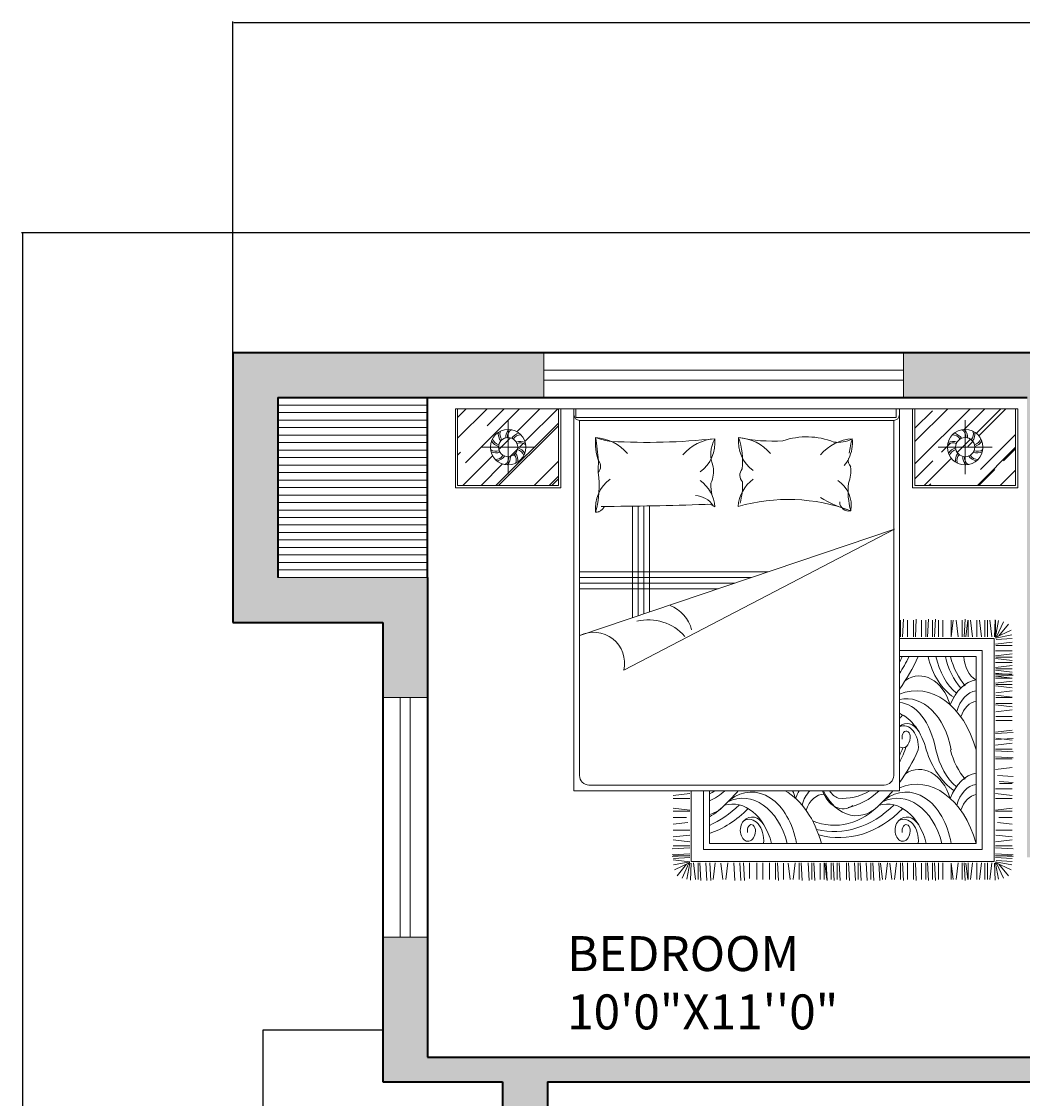
# Model space of a CAD drawing. Units: inches. Extents: x 2540 to 3167, y 3083 to 4007.
# Tile 12 of 15: x 2540 to 2741, y 3791 to 4007. Entities that reach past the tile are written whole.
import ezdxf

# ---------------------------------------------------------------- set-up
doc = ezdxf.new("R2010")
doc.units = ezdxf.units.IN
for name, color, linetype, lineweight in [('A-ANNO-DIMS', 2, 'Continuous', 18), ('A-AREA-IDEN', 7, 'Continuous', 18), ('A-FLOR-EDGE', 7, 'Continuous', 25), ('A-FLOR-PATT', 8, 'Continuous', 13), ('A-FURN', 8, 'Continuous', 13), ('A-GLAZ', 4, 'Continuous', 18)]:
    doc.layers.add(name, color=color, linetype=linetype, lineweight=lineweight)
doc.layers.add('A-WALL', color=143, linetype='Continuous', lineweight=35, true_color=0x7aafdf)
doc.layers.add('A-WALL-PATT', color=143, linetype='Continuous', lineweight=13, true_color=0x7aafdf)
doc.styles.get("Standard").update_dxf_attribs({"font": 'arial.ttf'})
doc.dimstyles.get("Standard").update_dxf_attribs({"dimtxt": 0.18, "dimasz": 0.18, "dimexe": 0.18, "dimexo": 0.0625, "dimgap": 0.09, "dimtad": 0, "dimtih": 1, "dimtoh": 1, "dimdec": 4, "dimzin": 0, "dimdsep": 46, "dimtxsty": 'Standard', "dimcen": 0.09, "dimadec": 0, "dimazin": 0, "dimtfac": 1, "dimtdec": 4, "dimtofl": 0, "dimtmove": 0, "dimatfit": 3, "dimfxl": 1, "dimtolj": 1, "dimtzin": 0, "dimarcsym": 0})

# ---------------------------------------------------------------- blocks, each defined once
blk = doc.blocks.new('*U1')
blk.add_line((0, 30), (0, 0))
blk = doc.blocks.new('*U2')
at = {"layer": 'A-FLOR-PATT', "color": 0, "linetype": 'ByBlock', "lineweight": -2, "transparency": 16777216, "rotation": 90}
for p in [(2621.51, 3931.71), (2621.51, 3930.21), (2621.51, 3928.71), (2621.51, 3927.21), (2621.51, 3925.71), (2621.51, 3924.21), (2621.51, 3922.71), (2621.51, 3921.21), (2621.51, 3919.71), (2621.51, 3918.21), (2621.51, 3916.71), (2621.51, 3915.21), (2621.51, 3913.71), (2621.51, 3912.21), (2621.51, 3910.71), (2621.51, 3909.21), (2621.51, 3907.71), (2621.51, 3906.21), (2621.51, 3904.71), (2621.51, 3903.21), (2621.51, 3901.71), (2621.51, 3900.21), (2621.51, 3898.71), (2621.51, 3897.21), (2621.51, 3895.71)]:
    blk.add_blockref('*U1', p, dxfattribs=at)
blk = doc.blocks.new('A$C64B41DC1')
for p, q in [((0, 2.5079), (2.9903, 2.5079)), ((0, 2.0879), (0, 2.5079)), ((0.012, 2.4618), (0.0581, 2.5079)), ((0.012, 2.3515), (0.1684, 2.5079)), ((0.012, 2.0999), (0.012, 2.5079)), ((0.0543, 2.2213), (0.3409, 2.5079)), ((0.1689, 2.4179), (0.2589, 2.5079)), ((0.3265, 2.386), (0.4484, 2.5079)), ((0.3699, 2.3332), (0.5445, 2.5079)), ((0.548, 2.5079), (0.548, 2.0999)), ((0.56, 2.5079), (0.56, 2.0879)), ((0.6301, 2.5079), (0.6301, 0.4779)), ((0.6401, 2.461), (0.6401, 2.5079)), ((0.6401, 2.5079), (2.344, 2.5079)), ((2.344, 2.5079), (2.3601, 2.5079)), ((2.344, 2.5079), (2.344, 2.461)), ((2.3601, 2.5079), (2.3601, 2.4761)), ((2.3601, 0.4779), (2.3601, 2.5079)), ((2.4303, 2.5079), (2.4303, 2.0879)), ((2.4423, 2.5079), (2.4423, 2.0999)), ((2.4423, 2.3333), (2.6169, 2.5079)), ((2.4423, 2.2145), (2.7357, 2.5079)), ((2.4423, 2.404), (2.5354, 2.4971)), ((2.705, 2.398), (2.8149, 2.5079)), ((2.7691, 2.3772), (2.8998, 2.5079)), ((2.7819, 2.3646), (2.9252, 2.5079)), ((2.9783, 2.0999), (2.9783, 2.5079)), ((2.9903, 2.0879), (2.9903, 2.5079)), ((0.2157, 2.0999), (0.548, 2.4322)), ((0.2299, 2.0999), (0.548, 2.418)), ((0.2804, 2.1597), (0.2804, 2.4481)), ((2.344, 2.461), (0.6401, 2.461)), ((0.6601, 2.4461), (1.4951, 2.4461)), ((0.6601, 2.4461), (0.6601, 0.5579)), ((1.4951, 2.4461), (0.6697, 2.4461)), ((2.3301, 2.4461), (1.4951, 2.4461)), ((2.3301, 0.5579), (2.3301, 2.4461)), ((2.7099, 2.1597), (2.7099, 2.4481)), ((0.2311, 2.2906), (0.2937, 2.3532)), ((2.7914, 2.1846), (2.9783, 2.3715)), ((0.1362, 2.3039), (0.4246, 2.3039)), ((0.2905, 2.2539), (0.3304, 2.2938)), ((0.3405, 2.3039), (0.3605, 2.3238)), ((2.8541, 2.3039), (2.5657, 2.3039)), ((2.5849, 2.2779), (2.6158, 2.3088)), ((2.6158, 2.3088), (2.6313, 2.3243)), ((2.6674, 2.2756), (2.7382, 2.3464)), ((2.7249, 2.3076), (2.7512, 2.3339)), ((2.7746, 2.0999), (2.9783, 2.3036)), ((2.9144, 2.2312), (2.9783, 2.2951)), ((0.012, 2.261), (0.0275, 2.2765)), ((0.0404, 2.0999), (0.1982, 2.2578)), ((2.4918, 2.0999), (2.6366, 2.2447)), ((0.1365, 2.0999), (0.251, 2.2144)), ((0.4194, 2.0999), (0.548, 2.2285)), ((2.4423, 2.1353), (2.5382, 2.2312)), ((2.7831, 2.0999), (2.8678, 2.1846)), ((2.8962, 2.0999), (2.9783, 2.182)), ((0.4986, 2.0999), (0.548, 2.1493)), ((0.5127, 2.0999), (0.548, 2.1352)), ((0.56, 2.0879), (0, 2.0879)), ((0.548, 2.0999), (0.012, 2.0999)), ((2.4303, 2.0879), (2.9903, 2.0879)), ((2.4423, 2.0999), (2.9783, 2.0999)), ((2.5172, 2.0999), (2.5269, 2.1096)), ((0.9415, 1.9902), (0.9415, 1.3975)), ((0.9715, 1.9906), (0.9715, 1.4076)), ((1.0015, 1.991), (1.0015, 1.4177)), ((1.0315, 1.9916), (1.0315, 1.4279)), ((2.3349, 1.8678), (0.6613, 1.3029)), ((0.8956, 1.1191), (2.3349, 1.8678)), ((1.6636, 1.6412), (0.6601, 1.6412)), ((1.5748, 1.6112), (0.6601, 1.6112)), ((2.3665, 1.295), (2.3665, 1.3839)), ((2.377, 1.295), (2.3822, 1.3891)), ((2.4032, 1.295), (2.4032, 1.3839)), ((2.4346, 1.295), (2.4346, 1.3839)), ((2.4451, 1.295), (2.4503, 1.3891)), ((2.4774, 1.2957), (2.4774, 1.3837)), ((2.5, 1.295), (2.5, 1.3839)), ((2.5105, 1.295), (2.5157, 1.3891)), ((2.5367, 1.295), (2.5367, 1.3839)), ((2.5471, 1.295), (2.5524, 1.3891)), ((2.5681, 1.295), (2.5681, 1.3839)), ((2.5918, 1.295), (2.5918, 1.3839)), ((2.6346, 1.2957), (2.6346, 1.3837)), ((2.6362, 1.2957), (2.6467, 1.3839)), ((2.6729, 1.295), (2.6624, 1.3839)), ((2.6938, 1.295), (2.6938, 1.3839)), ((2.7043, 1.295), (2.7095, 1.3891)), ((2.7127, 1.2957), (2.7232, 1.3839)), ((2.7253, 1.295), (2.7253, 1.3839)), ((2.7494, 1.295), (2.7389, 1.3839)), ((2.7718, 1.295), (2.7718, 1.3839)), ((2.7959, 1.295), (2.7854, 1.3839)), ((2.8146, 1.2957), (2.8146, 1.3837)), ((2.8146, 1.2957), (2.8146, 1.3837)), ((2.8282, 1.295), (2.8282, 1.3839)), ((2.8282, 1.295), (2.8282, 1.3839)), ((2.8523, 1.295), (2.8418, 1.3839)), ((2.8523, 1.295), (2.8418, 1.3839)), ((2.8653, 1.2966), (2.8688, 1.3861)), ((2.8711, 1.2957), (2.8711, 1.3837)), ((2.8711, 1.2957), (2.8875, 1.3822)), ((2.8765, 1.2958), (2.9132, 1.3758)), ((2.8713, 1.2927), (2.954, 1.3315)), ((2.8893, 1.3011), (2.9394, 1.3636)), ((2.3601, 1.2873), (2.8639, 1.2873)), ((2.8639, 1.2873), (2.8639, 0.1018)), ((2.8716, 1.2565), (2.9605, 1.2669)), ((2.8717, 1.2884), (2.9588, 1.3058)), ((2.8744, 1.2817), (2.9603, 1.2869)), ((2.3601, 1.2233), (2.7999, 1.2233)), ((2.7999, 1.2233), (2.7999, 0.1658)), ((2.8716, 1.2212), (2.9605, 1.2212)), ((2.8716, 1.1947), (2.9605, 1.2052)), ((2.8723, 1.2489), (2.9603, 1.2489)), ((2.3601, 1.1913), (2.7679, 1.1912)), ((2.7679, 1.1912), (2.7679, 0.1978)), ((2.8716, 1.181), (2.9605, 1.1705)), ((2.8716, 1.1595), (2.9605, 1.1595)), ((2.8723, 1.1872), (2.9603, 1.1872)), ((2.8716, 1.133), (2.9605, 1.1435)), ((2.8716, 1.1193), (2.9605, 1.1088)), ((2.8716, 1.1035), (2.9605, 1.093)), ((2.8716, 1.0965), (2.9605, 1.0965)), ((2.8716, 1.086), (2.9657, 1.0913)), ((2.8723, 1.1255), (2.9603, 1.1255)), ((2.8716, 1.0756), (2.9605, 1.0756)), ((2.8716, 1.0491), (2.9605, 1.0596)), ((2.8716, 1.0354), (2.9605, 1.0249)), ((2.8723, 1.0858), (2.9605, 1.0753)), ((2.8723, 1.0416), (2.9603, 1.0416)), ((2.8723, 0.9987), (2.9605, 1.0092)), ((2.8723, 0.985), (2.9605, 0.9745)), ((2.8723, 0.9735), (2.9603, 0.9735)), ((2.8716, 0.9346), (2.9605, 0.9241)), ((2.8723, 0.9408), (2.9603, 0.9408)), ((2.8723, 0.8979), (2.9605, 0.9084)), ((2.8723, 0.8726), (2.9603, 0.8726)), ((2.8723, 0.8505), (2.9603, 0.8505)), ((2.8716, 0.7885), (2.9605, 0.799)), ((2.8716, 0.7818), (2.9657, 0.787)), ((2.8716, 0.7503), (2.9657, 0.7556)), ((2.8723, 0.7571), (2.9605, 0.7466)), ((2.8716, 0.7204), (2.9605, 0.7309)), ((2.8716, 0.6995), (2.9605, 0.6995)), ((2.8716, 0.689), (2.9657, 0.6838)), ((2.8716, 0.6576), (2.9657, 0.6523)), ((2.8716, 0.6471), (2.9605, 0.6471)), ((2.8716, 0.5903), (2.9605, 0.6007)), ((2.882, 0.5582), (2.9657, 0.5536)), ((2.8909, 0.5263), (2.9657, 0.5222)), ((2.8928, 0.5169), (2.9605, 0.5169)), ((0.6301, 0.4779), (2.3601, 0.4779)), ((0.7101, 0.5079), (2.2801, 0.5079)), ((1.2465, 0.4625), (1.1576, 0.452)), ((1.2542, 0.1018), (1.2542, 0.4779)), ((1.3182, 0.1658), (1.3182, 0.4779)), ((1.3502, 0.1978), (1.3502, 0.4779)), ((2.8716, 0.4877), (2.9603, 0.4877)), ((2.8716, 0.4625), (2.9605, 0.452)), ((1.2465, 0.4365), (1.1577, 0.4365)), ((2.8716, 0.4365), (2.9603, 0.4365)), ((1.2465, 0.3746), (1.1576, 0.3851)), ((1.2465, 0.3684), (1.1577, 0.3684)), ((2.8716, 0.3746), (2.9605, 0.3851)), ((2.8716, 0.3684), (2.9603, 0.3684)), ((1.2355, 0.3092), (1.1576, 0.3)), ((1.2285, 0.3357), (1.1577, 0.3357)), ((2.8826, 0.3092), (2.9605, 0.3)), ((2.8896, 0.3357), (2.9603, 0.3357)), ((1.2457, 0.2423), (1.1576, 0.2319)), ((1.2457, 0.2676), (1.1577, 0.2676)), ((2.8723, 0.2676), (2.9603, 0.2676)), ((2.8723, 0.2423), (2.9605, 0.2319)), ((1.2465, 0.1742), (1.1524, 0.169)), ((1.2465, 0.2057), (1.1576, 0.2161)), ((1.2465, 0.1847), (1.1576, 0.1847)), ((2.7679, 0.1978), (1.3502, 0.1978)), ((2.8716, 0.2057), (2.9605, 0.2161)), ((2.8716, 0.1847), (2.9605, 0.1847)), ((2.8716, 0.1742), (2.9657, 0.169)), ((1.2465, 0.1428), (1.1524, 0.1376)), ((1.2465, 0.1334), (1.1524, 0.1281)), ((1.2465, 0.1323), (1.1576, 0.1323)), ((1.2465, 0.1323), (1.1576, 0.1323)), ((1.2465, 0.1229), (1.1588, 0.1168)), ((2.7999, 0.1658), (1.3182, 0.1658)), ((2.8716, 0.1428), (2.9657, 0.1376)), ((2.8716, 0.1334), (2.9657, 0.1281)), ((2.8716, 0.1323), (2.9605, 0.1323)), ((2.8716, 0.1229), (2.9593, 0.1168)), ((1.2465, 0.1), (1.1576, 0.1105)), ((1.2464, 0.1007), (1.1592, 0.0833)), ((1.2468, 0.0964), (1.1641, 0.0576)), ((1.2288, 0.088), (1.1787, 0.0255)), ((1.2415, 0.0933), (1.2049, 0.0133)), ((1.247, 0.0934), (1.2306, 0.0069)), ((1.2527, 0.0925), (1.2493, 0.003)), ((2.8639, 0.1018), (1.2542, 0.1018)), ((1.2658, 0.0941), (1.2762, 0.0052)), ((1.2899, 0.0941), (1.2899, 0.0052)), ((1.2999, 0.0941), (1.3051, 0)), ((1.3313, 0.0941), (1.3365, 0)), ((1.3523, 0.0941), (1.3575, 0)), ((1.3804, 0.0941), (1.3699, 0.0052)), ((1.4119, 0.0934), (1.4223, 0.0052)), ((1.4485, 0.0941), (1.438, 0.0052)), ((1.48, 0.0941), (1.4852, 0)), ((1.5114, 0.0941), (1.5166, 0)), ((1.5323, 0.0941), (1.5376, 0)), ((1.5638, 0.0941), (1.5638, 0.0105)), ((1.6021, 0.0941), (1.6021, 0.0052)), ((1.6336, 0.0941), (1.6336, 0.0052)), ((1.6702, 0.0941), (1.6702, 0.0052)), ((1.7017, 0.0941), (1.7017, 0.0052)), ((1.7122, 0.0941), (1.7174, 0)), ((1.7445, 0.0934), (1.7445, 0.0054)), ((1.7698, 0.0934), (1.7803, 0.0052)), ((1.8065, 0.0941), (1.796, 0.0052)), ((1.8274, 0.0941), (1.8274, 0.0052)), ((1.8379, 0.0941), (1.8431, 0)), ((1.8746, 0.0941), (1.8798, 0)), ((1.8955, 0.0941), (1.8955, 0.0052)), ((1.906, 0.0941), (1.9113, 0)), ((1.9384, 0.0934), (1.9384, 0.0054)), ((1.9609, 0.0941), (1.9609, 0.0052)), ((1.9636, 0.0934), (1.9741, 0.0052)), ((1.9714, 0.0941), (1.9766, 0)), ((1.9976, 0.0941), (1.9976, 0.0052)), ((2.0081, 0.0941), (2.0133, 0)), ((2.029, 0.0941), (2.029, 0.0052)), ((2.0395, 0.0941), (2.0447, 0)), ((2.0797, 0.0941), (2.0797, 0.0052)), ((2.0902, 0.0941), (2.0954, 0)), ((2.1216, 0.0941), (2.1269, 0)), ((2.1412, 0.0941), (2.1412, 0.0052)), ((2.1517, 0.0941), (2.1569, 0)), ((2.1831, 0.0941), (2.1884, 0)), ((2.2093, 0.0941), (2.2093, 0.0052)), ((2.2198, 0.0941), (2.225, 0)), ((2.2512, 0.0941), (2.2565, 0)), ((2.2603, 0.0934), (2.2707, 0.0052)), ((2.2969, 0.0941), (2.2864, 0.0052)), ((2.3089, 0.0934), (2.3193, 0.0052)), ((2.3455, 0.0941), (2.3351, 0.0052)), ((2.3665, 0.0941), (2.3665, 0.0052)), ((2.377, 0.0941), (2.3822, 0)), ((2.4032, 0.0941), (2.4032, 0.0052)), ((2.4346, 0.0941), (2.4346, 0.0052)), ((2.4451, 0.0941), (2.4503, 0)), ((2.4774, 0.0934), (2.4774, 0.0054)), ((2.5, 0.0941), (2.5, 0.0052)), ((2.5105, 0.0941), (2.5157, 0)), ((2.5367, 0.0941), (2.5367, 0.0052)), ((2.5471, 0.0941), (2.5524, 0)), ((2.5681, 0.0941), (2.5681, 0.0052)), ((2.5918, 0.0941), (2.5918, 0.0052)), ((2.6346, 0.0934), (2.6346, 0.0054)), ((2.6362, 0.0934), (2.6467, 0.0052)), ((2.6729, 0.0941), (2.6624, 0.0052)), ((2.6938, 0.0941), (2.6938, 0.0052)), ((2.7043, 0.0941), (2.7095, 0)), ((2.7127, 0.0934), (2.7232, 0.0052)), ((2.7253, 0.0941), (2.7253, 0.0052)), ((2.7494, 0.0941), (2.7389, 0.0052)), ((2.7718, 0.0941), (2.7718, 0.0052)), ((2.7959, 0.0941), (2.7854, 0.0052)), ((2.8146, 0.0934), (2.8146, 0.0054)), ((2.8282, 0.0941), (2.8282, 0.0052)), ((2.8523, 0.0941), (2.8418, 0.0052)), ((2.8653, 0.0925), (2.8688, 0.003)), ((2.8711, 0.0934), (2.8875, 0.0069)), ((2.8713, 0.0964), (2.954, 0.0576)), ((2.8717, 0.1007), (2.9588, 0.0833)), ((2.8744, 0.1074), (2.9603, 0.1022)), ((2.8765, 0.0933), (2.9132, 0.0133)), ((2.8893, 0.088), (2.9394, 0.0255))]:
    blk.add_line(p, q)
at = {"ltscale": 10}
for p, q in [((1.4859, 1.5812), (0.6601, 1.5812)), ((1.397, 1.5512), (0.6601, 1.5512))]:
    blk.add_line(p, q, dxfattribs=at)
for centre, radius in [((0.2804, 2.3039), 0.0942), ((0.2804, 2.3039), 0.051), ((2.7099, 2.3039), 0.0942), ((2.7099, 2.3039), 0.051)]:
    blk.add_circle(centre, radius)
for centre, radius, start, end in [((0.6601, 2.4761), 0.03, 180, 270), ((2.3301, 2.4761), 0.03, 270, 0), ((0.2417, 2.3614), 0.0462, 196.3002, 256.538), ((0.2887, 2.3745), 0.0605, 172.17, 218.4897), ((0.2828, 2.3731), 0.0462, 160.3002, 220.538), ((0.3286, 2.3561), 0.0605, 136.17, 182.4897), ((0.3231, 2.3585), 0.0462, 124.3002, 184.538), ((0.3501, 2.3178), 0.0605, 100.17, 146.4897), ((0.347, 2.323), 0.0462, 88.3002, 148.538), ((1.0526, 2.3302), 0.3085, 175.3048, 198.6942), ((-0.8702, 2.0941), 1.6364, 4.8098, 9.1892), ((0.8579, 2.6278), 0.2948, 247.5179, 264.267), ((0.728, 2.111), 0.245, 40.4189, 85.9871), ((1.0164, 5.7096), 3.3803, 266.8134, 276.1602), ((1.3963, 2.1044), 0.245, 94.0129, 139.5811), ((1.1858, 2.3288), 0.1943, 306.5711, 5.89), ((1.5348, 2.2652), 0.1767, 151.7736, 201.6983), ((1.6986, 2.3355), 0.1943, 174.11, 233.4289), ((1.1481, 2.2311), 0.3783, 353.4947, 19.1867), ((1.6871, 3.192), 0.8561, 257.7438, 273.6284), ((1.4882, 2.111), 0.245, 40.4189, 85.9871), ((1.8674, 1.9709), 0.3878, 68.2026, 108.9817), ((2.1269, 2.1044), 0.245, 94.0129, 139.5811), ((2.0342, 2.4856), 0.1563, 261.5958, 298.9092), ((1.9165, 2.3288), 0.1943, 333.7371, 5.89), ((2.6058, 2.2028), 0.517, 163.6046, 172.3273), ((2.6433, 2.323), 0.0462, 31.462, 91.6998), ((2.6402, 2.3178), 0.0605, 33.5103, 79.83), ((2.6672, 2.3585), 0.0462, 355.462, 55.6998), ((2.6617, 2.3561), 0.0605, 357.5103, 43.83), ((2.7075, 2.3731), 0.0462, 319.462, 19.6998), ((2.7016, 2.3745), 0.0605, 321.5103, 7.83), ((2.7486, 2.3614), 0.0462, 283.462, 343.6998), ((0.2153, 2.3276), 0.0462, 232.3002, 292.538), ((0.2457, 2.3659), 0.0605, 208.17, 254.4897), ((0.3449, 2.2742), 0.0605, 64.17, 110.4897), ((0.3455, 2.2802), 0.0462, 52.3002, 112.538), ((0.3191, 2.2464), 0.0462, 16.3002, 76.538), ((0.3151, 2.2419), 0.0605, 28.17, 74.4897), ((2.6448, 2.2802), 0.0462, 67.462, 127.6998), ((2.6454, 2.2742), 0.0605, 69.5103, 115.83), ((2.6752, 2.2419), 0.0605, 105.5103, 151.83), ((2.6712, 2.2464), 0.0462, 103.462, 163.6998), ((2.775, 2.3276), 0.0462, 247.462, 307.6998), ((2.7446, 2.3659), 0.0605, 285.5103, 331.83), ((0.2158, 2.3336), 0.0605, 244.17, 290.4897), ((0.2138, 2.2848), 0.0462, 268.3002, 328.538), ((0.2107, 2.29), 0.0605, 280.17, 326.4897), ((0.2377, 2.2493), 0.0462, 304.3002, 4.538), ((0.2322, 2.2517), 0.0605, 316.17, 2.4897), ((0.2779, 2.2347), 0.0462, 340.3002, 40.538), ((0.272, 2.2333), 0.0605, 352.17, 38.4897), ((1.9165, 2.3288), 0.1943, 320.9404, 333.7371), ((2.1347, 2.2313), 0.0459, 165.3506, 223.2684), ((2.7182, 2.2333), 0.0605, 141.5103, 187.83), ((2.7123, 2.2347), 0.0462, 139.462, 199.6998), ((2.7581, 2.2517), 0.0605, 177.5103, 223.83), ((2.7526, 2.2493), 0.0462, 175.462, 235.6998), ((2.7796, 2.29), 0.0605, 213.5103, 259.83), ((2.7765, 2.2848), 0.0462, 211.462, 271.6998), ((2.7744, 2.3336), 0.0605, 249.5103, 295.83), ((0.7274, 2.2013), 0.0446, 314.4736, 42.1713), ((-1.6008, 2.277), 2.3618, 357.3905, 358.8876), ((1.204, 2.1778), 0.1681, 337.017, 7.5368), ((1.5671, 2.1546), 0.0547, 142.0833, 220.902), ((1.9346, 2.1778), 0.1681, 337.017, 7.5368), ((0.9385, 1.978), 0.1943, 126.5711, 185.89), ((0.2688, 2.0945), 0.4956, 344.0243, 8.7071), ((1.1858, 1.9714), 0.1943, 4.3181, 53.4289), ((1.7059, 1.9714), 0.204, 127.1197, 175.09), ((1.1965, 2.0983), 0.3299, 343.7954, 3.5554), ((1.9394, 1.991), 0.1651, 351.2621, 55.7572), ((1.5415, 2.0969), 0.1834, 175.2233, 196.23), ((2.4617, 2.0719), 0.3745, 173.8296, 196.4356), ((1.2687, 1.9248), 0.1223, 33.628, 86.4744), ((1.7676, 1.0629), 0.9631, 69.6507, 105.9631), ((2.2748, 2.5795), 0.6373, 238.3499, 254.3137), ((2.0911, 2.0123), 0.0478, 179.7727, 283.8018), ((0.7417, 2.0149), 0.057, 273.4709, 328.5412), ((0.728, 2.2025), 0.245, 274.0129, 278.3417), ((0.7246, 18.8439), 16.8552, 270.17399, 272.05214), ((1.3401, 1.9404), 0.0603, 49.0991, 101.3702), ((1.0747, 1.2871), 0.1871, 14.1863, 69.1212), ((1.0274, 1.1334), 0.2527, 40.629, 104.3712), ((0.7347, 1.1553), 0.1649, 347.3109, 116.4454), ((0.7101, 0.5579), 0.05, 180, 270), ((2.2801, 0.5579), 0.05, 270, 0)]:
    blk.add_arc(centre, radius, start, end)
for centre, major_axis, ratio, start_param, end_param in [((1.9938, 1.6262), (0, -0.7531), 0.68, 0.797284, 0.954936), ((2.0643, 1.466), (0, -0.5322), 0.68, 7.239912, 7.311536), ((1.9052, 1.7397), (0, -0.9842), 0.68, 0.74745, 0.979724), ((2.7455, 1.3081), (0, 0.3614), 0.68, 1.900046, 2.742661), ((2.7868, 1.3081), (0, 0.3614), 0.68, 1.900046, 2.614747), ((2.8372, 1.3081), (0, 0.3614), 0.68, 1.900046, 2.479658), ((2.8607, 1.3211), (0, 0.3614), 0.68, 1.938265, 2.479658), ((2.8057, 1.2079), (0, -0.1524), 0.68, 4.821745, 5.895886), ((2.4665, 0.8216), (0, -0.2664), 0.68, 2.006169, 3.565187), ((2.4513, 0.5069), (0, 0.502), 0.68, 5.095327, 6.553458), ((2.7862, 0.8069), (0, -0.2615), 0.68, 3.244645, 4.205018), ((2.396, 0.6032), (0, 0.3641), 0.68, -1.3172, 0.145284), ((2.7784, 0.8289), (0, -0.1802), 0.68, 3.227058, 4.318474), ((2.3507, 0.5642), (0.0073, 0.3819), 0.56205, -1.21172, -0.009991), ((2.7821, 0.7971), (0, -0.1589), 0.68, 3.272942, 4.229533), ((2.2964, 0.5771), (0, -0.3263), 0.68, 1.938944, 2.850232), ((2.0403, 1.6015), (0, -0.8763), 0.68, 6.849801, 6.887077), ((2.4005, 0.7132), (0, -0.1214), 0.68, 2.284368, 3.652258), ((2.3834, 0.7081), (0, 0.1147), 0.68, 4.593909, 6.585576), ((2.3774, 0.7653), (0, -0.0593), 0.68, 5.841311, 7.755362), ((2.3961, 0.7628), (0, -0.0317), 0.68, 1.462497, 5.046281), ((1.9938, 1.1295), (-0.0678, 0.7439), 0.610498, 3.917146, 4.063997), ((2.0643, 0.9693), (0, -0.5322), 0.68, 7.239912, 7.336618), ((1.9052, 1.243), (0, -0.9842), 0.68, 0.74745, 0.979724), ((2.7455, 0.8114), (-0.0599, 0.3735), 0.695517, 1.775813, 2.548612), ((2.7868, 0.8114), (0, 0.3614), 0.68, 1.900046, 2.614747), ((2.8607, 0.8243), (0, 0.3614), 0.68, 1.938265, 2.479658), ((2.4665, 0.3249), (0, -0.2664), 0.68, 2.006169, 3.565187), ((2.4513, 0.0102), (0, 0.502), 0.68, 5.095327, 6.553458), ((2.7862, 0.3102), (0, -0.2615), 0.68, 3.244645, 4.205018), ((1.242, 0.9693), (0, -0.5322), 0.68, 6.586764, 6.677612), ((1.1714, 1.1295), (-0.1157, 0.7241), 0.59432, 3.291697, 3.50733), ((1.0828, 1.243), (0, -0.9842), 0.68, 0.565948, 0.680366), ((1.5283, 0.0674), (0, -0.3703), 0.68, 1.930561, 3.464283), ((1.5736, 0.1065), (0, 0.3641), 0.68, -1.3172, 0.476403), ((1.6289, 0.0102), (0, 0.502), 0.68, 6.655152, 6.661293), ((1.6289, 0.0102), (0, 0.502), 0.68, 5.095327, 5.911219), ((1.6442, 0.3249), (0, -0.2664), 0.68, 2.006169, 2.182797), ((1.9638, 0.3102), (0, -0.2615), 0.68, 4.015924, 4.205018), ((1.956, 0.3322), (0, -0.1802), 0.68, 3.770744, 4.318474), ((1.9597, 0.3004), (0, -0.1589), 0.68, 3.14258, 4.229533), ((2.0606, 0.5616), (0, -0.1803), 0.68, 5.194792, 5.929328), ((2.0606, 0.5616), (0, -0.1803), 0.68, 5.194792, 6.723255), ((2.1315, 0.6603), (0, -0.3155), 0.68, 5.328638, 6.949396), ((2.0549, 0.5656), (0, -0.1303), 0.68, 5.450951, 6.054641), ((2.0643, 0.9693), (0, -0.5322), 0.68, 6.20013, 6.677612), ((1.9938, 1.1295), (-0.0678, 0.7439), 0.610498, 3.199135, 3.592282), ((1.9052, 1.243), (0, -0.9842), 0.68, 0.565948, 0.680366), ((2.3507, 0.0674), (0, -0.3703), 0.68, 1.930561, 3.464283), ((2.396, 0.1065), (0, 0.3641), 0.68, -1.3172, 0.476403), ((2.4513, 0.0102), (0, 0.502), 0.68, 6.655152, 6.661293), ((2.7784, 0.3322), (0, -0.1802), 0.68, 3.227058, 4.318474), ((2.7821, 0.3004), (0, -0.1589), 0.68, 3.272942, 4.229533), ((1.1933, 0.9181), (0, -0.624), 0.68, 0.378672, 0.625379), ((1.3091, 0.6603), (0, -0.3155), 0.68, 6.475719, 6.949396), ((1.1911, 1.1066), (0, 0.8458), 0.68, 3.421828, 3.728616), ((1.474, 0.0804), (0, -0.3263), 0.68, 1.938944, 3.339184), ((2.0157, 0.9181), (0, -0.624), 0.68, -0.280078, 0.625379), ((2.0135, 1.1066), (0, 0.8458), 0.68, 2.978727, 3.728616), ((2.2964, 0.0804), (0, -0.3263), 0.68, 1.938944, 3.339184), ((1.2179, 1.1047), (0, -0.8763), 0.68, 6.507006, 6.887077), ((1.5781, 0.2165), (0, -0.1214), 0.68, 2.284368, 3.726131), ((2.0403, 1.1047), (0, -0.8763), 0.68, 6.099302, 6.887077), ((2.4005, 0.2165), (0, -0.1214), 0.68, 2.284368, 3.726131), ((1.555, 0.2685), (0, -0.0593), 0.68, 3.732151, 7.755362), ((1.561, 0.2114), (0, 0.1147), 0.68, 4.593909, 6.647252), ((1.5737, 0.2661), (0, -0.0317), 0.68, 1.462497, 5.046281), ((2.3774, 0.2685), (0, -0.0593), 0.68, 3.732151, 7.755362), ((2.3834, 0.2114), (0, 0.1147), 0.68, 4.593909, 6.647252), ((2.3961, 0.2661), (0, -0.0317), 0.68, 1.462497, 5.046281)]:
    blk.add_ellipse(centre, major_axis=major_axis, ratio=ratio, start_param=start_param, end_param=end_param)
blk = doc.blocks.new('WIN-48IN')
for p, q in [((0, 48), (9, 48)), ((3.5, 0), (3.5, 48)), ((5.5, 0), (5.5, 48)), ((0, 0), (9, 0))]:
    blk.add_line(p, q)
blk = doc.blocks.new('WIN-72IN')
for p, q in [((9, 72), (0, 72)), ((3.5, 0), (3.5, 72)), ((5.5, 0), (5.5, 72)), ((9, 0), (0, 0))]:
    blk.add_line(p, q)
blk = doc.blocks.new('*D43')
at = {"layer": 'A-ANNO-DIMS', "color": 0, "lineweight": -2, "transparency": 16777216}
for p, q in [((2582.51, 3940.78), (2582.51, 4006.99)), ((2582.69, 4006.81), (2853.22, 4006.81)), ((3124.33, 4006.81), (2853.8, 4006.81)), ((3124.51, 3940.78), (3124.51, 4006.99))]:
    blk.add_line(p, q, dxfattribs=at)
at = {"layer": 'A-ANNO-DIMS', "color": 0, "transparency": 16777216}
for points in [[(2582.69, 4006.84), (2582.69, 4006.78), (2582.51, 4006.81)], [(3124.33, 4006.84), (3124.33, 4006.78), (3124.51, 4006.81)]]:
    blk.add_solid(points, dxfattribs=at)
at = {"layer": 'Defpoints', "color": 0, "transparency": 16777216}
for p in [(3124.51, 4006.81), (2582.51, 3940.71), (3124.51, 3940.71)]:
    blk.add_point(p, dxfattribs=at)
at = {"layer": 'A-ANNO-DIMS', "color": 0, "transparency": 16777216, "insert": (2853.51, 4006.81), "char_height": 0.18, "attachment_point": 5}
blk.add_mtext('\\A1;542', dxfattribs=at)
blk = doc.blocks.new('*D44')
at = {"layer": 'A-ANNO-DIMS', "color": 0, "lineweight": -2, "transparency": 16777216}
for p, q in [((2771.45, 3964.71), (2540.23, 3964.71)), ((2540.41, 3964.53), (2540.41, 3545.4)), ((2540.41, 3125.89), (2540.41, 3545.03)), ((2810.45, 3125.71), (2540.23, 3125.71))]:
    blk.add_line(p, q, dxfattribs=at)
at = {"layer": 'A-ANNO-DIMS', "color": 0, "transparency": 16777216}
for points in [[(2540.38, 3964.53), (2540.44, 3964.53), (2540.41, 3964.71)], [(2540.38, 3125.89), (2540.44, 3125.89), (2540.41, 3125.71)]]:
    blk.add_solid(points, dxfattribs=at)
at = {"layer": 'Defpoints', "color": 0, "transparency": 16777216}
for p in [(2540.41, 3964.71), (2771.51, 3964.71), (2810.51, 3125.71)]:
    blk.add_point(p, dxfattribs=at)
at = {"layer": 'A-ANNO-DIMS', "color": 0, "transparency": 16777216, "insert": (2540.41, 3545.21), "char_height": 0.18, "attachment_point": 5}
blk.add_mtext('\\A1;839', dxfattribs=at)

msp = doc.modelspace()

# ---------------------------------------------------------------- hatches: boundary and pattern name
at = {"layer": 'A-WALL-PATT'}
h = msp.add_hatch(color=256, dxfattribs=at)
h.dxf.hatch_style = 1
h.paths.add_polyline_path([(2644.77, 3940.71), (2582.51, 3940.71), (2582.51, 3886.71), (2612.51, 3886.71), (2612.51, 3871.71), (2621.51, 3871.71), (2621.51, 3895.71), (2591.51, 3895.71), (2591.51, 3931.71), (2621.51, 3931.71), (2644.77, 3931.71)])
h.paths.add_polyline_path([(2746.51, 3940.71), (2716.77, 3940.71), (2716.77, 3931.71), (2741.51, 3931.71), (2741.51, 3839.71), (2748.51, 3839.71), (2748.51, 3844.71), (2746.51, 3844.71), (2746.51, 3931.71)])
h.paths.add_polyline_path([(2805.51, 3959.71), (2925.51, 3959.71), (2925.51, 3916.71), (2913.51, 3916.71), (2913.51, 3907.71), (2925.51, 3907.71), (2925.51, 3880.71), (2930.51, 3880.71), (2930.51, 3931.71), (2978.28, 3931.71), (2978.28, 3940.71), (2930.51, 3940.71), (2930.51, 3964.71), (2800.51, 3964.71), (2800.51, 3940.71), (2776.51, 3940.71), (2776.51, 3964.71), (2771.51, 3964.71), (2771.51, 3940.71), (2771.51, 3931.71), (2800.51, 3931.71), (2800.51, 3839.71), (2805.51, 3839.71), (2805.51, 3907.71), (2817.48, 3907.71), (2817.48, 3916.71), (2805.51, 3916.71)])
h.paths.add_polyline_path([(3124.51, 3940.71), (3026.28, 3940.71), (3026.28, 3931.71), (3062.51, 3931.71), (3062.51, 3924.21), (3071.51, 3924.21), (3071.51, 3931.71), (3119.51, 3931.71), (3119.51, 3832.71), (2925.51, 3832.71), (2925.51, 3815.71), (2930.51, 3815.71), (2930.51, 3827.71), (2976.51, 3827.71), (2976.51, 3773.71), (2970.51, 3773.71), (2970.51, 3768.71), (2985.51, 3768.71), (2985.51, 3773.71), (2981.51, 3773.71), (2981.51, 3827.71), (3086.51, 3827.71), (3086.51, 3812.71), (3095.51, 3812.71), (3095.51, 3827.71), (3124.51, 3827.71)])
h = msp.add_hatch(color=256, dxfattribs=at)
h.dxf.hatch_style = 1
h.paths.add_polyline_path([(2805.51, 3803.71), (2800.51, 3803.71), (2800.51, 3799.71), (2621.51, 3799.71), (2621.51, 3823.71), (2612.51, 3823.71), (2612.51, 3794.71), (2636.51, 3794.71), (2636.51, 3782.71), (2645.51, 3782.71), (2645.51, 3794.71), (2805.51, 3794.71)])
h.paths.add_polyline_path([(2810.51, 3564.71), (2868.51, 3564.71), (2868.51, 3627.71), (2872.51, 3627.71), (2872.51, 3636.71), (2864.51, 3636.71), (2864.51, 3674.71), (2797.51, 3674.71), (2797.51, 3669.71), (2801.51, 3669.71), (2801.51, 3628.63), (2806.51, 3628.63), (2806.51, 3669.71), (2859.51, 3669.71), (2859.51, 3573.71), (2806.51, 3573.71), (2806.51, 3598.63), (2801.51, 3598.63), (2801.51, 3549.71), (2645.51, 3549.71), (2645.51, 3573.71), (2636.51, 3573.71), (2636.51, 3516.71), (2645.51, 3516.71), (2645.51, 3540.71), (2801.51, 3540.71), (2801.51, 3504.71), (2801.51, 3500.71), (2806.51, 3500.71), (2806.51, 3504.71), (2859.51, 3504.71), (2859.51, 3420.71), (2806.51, 3420.71), (2806.51, 3470.71), (2801.51, 3470.71), (2801.51, 3420.71), (2797.51, 3420.71), (2797.51, 3415.71), (2864.51, 3415.71), (2864.51, 3453.71), (2868.51, 3453.71), (2868.51, 3513.71), (2810.51, 3513.71)])
h.paths.add_polyline_path([(2645.51, 3415.71), (2761.51, 3415.71), (2761.51, 3420.71), (2645.51, 3420.71), (2645.51, 3444.71), (2636.51, 3444.71), (2636.51, 3403.71), (2645.51, 3403.71)])
h.paths.add_polyline_path([(2645.51, 3307.71), (2636.51, 3307.71), (2636.51, 3295.71), (2612.51, 3295.71), (2612.51, 3149.71), (2645.51, 3149.71), (2645.51, 3158.71), (2621.51, 3158.71), (2621.51, 3290.71), (2801.51, 3290.71), (2801.51, 3286.71), (2806.51, 3286.71), (2806.51, 3295.71), (2645.51, 3295.71)])
h.paths.add_polyline_path([(2762.01, 3158.71), (2746.51, 3158.71), (2746.51, 3240.71), (2750.51, 3240.71), (2750.51, 3245.71), (2741.51, 3245.71), (2741.51, 3158.71), (2717.51, 3158.71), (2717.51, 3149.71), (2762.01, 3149.71)], flags=17)
h.paths.add_polyline_path([(2810.51, 3173.71), (2822.51, 3173.71), (2822.51, 3182.71), (2806.51, 3182.71), (2806.51, 3250.71), (2801.51, 3250.71), (2801.51, 3245.71), (2780.51, 3245.71), (2780.51, 3240.71), (2801.51, 3240.71), (2801.51, 3158.71), (2786.01, 3158.71), (2786.01, 3149.71), (2810.51, 3149.71)])
h.paths.add_polyline_path([(2931.51, 3290.71), (2935.51, 3290.71), (2935.51, 3295.71), (2926.51, 3295.71), (2926.51, 3182.71), (2910.51, 3182.71), (2910.51, 3173.71), (2922.51, 3173.71), (2922.51, 3149.71), (2987.51, 3149.71), (2987.51, 3158.71), (2931.51, 3158.71)])
h.paths.add_polyline_path([(3124.51, 3295.71), (3086.51, 3295.71), (3018.51, 3295.71), (3018.51, 3290.71), (3115.51, 3290.71), (3115.51, 3158.71), (3059.51, 3158.71), (3059.51, 3149.71), (3124.51, 3149.71)])
h.paths.add_polyline_path([(2988.51, 3295.71), (2984.51, 3295.71), (2984.51, 3349.71), (3086.51, 3349.71), (3086.51, 3320.71), (3124.51, 3320.71), (3124.51, 3354.71), (3071.51, 3354.71), (3071.51, 3358.71), (3062.51, 3358.71), (3062.51, 3354.71), (2979.51, 3354.71), (2979.51, 3295.71), (2971.51, 3295.71), (2971.51, 3290.71), (2988.51, 3290.71)])
h.paths.add_polyline_path([(3095.51, 3325.71), (3095.51, 3349.71), (3119.51, 3349.71), (3119.51, 3325.71)], flags=16)
h.paths.add_polyline_path([(3124.51, 3462.71), (3071.51, 3462.71), (3071.51, 3627.71), (3124.51, 3627.71), (3124.51, 3693.71), (3095.51, 3693.71), (3095.51, 3702.71), (3086.51, 3702.71), (3086.51, 3684.71), (3086.51, 3636.71), (2930.51, 3636.71), (2930.51, 3768.71), (2934.51, 3768.71), (2934.51, 3773.71), (2930.51, 3773.71), (2925.51, 3773.71), (2925.51, 3730.71), (2864.51, 3730.71), (2864.51, 3760.71), (2859.51, 3760.71), (2859.51, 3725.71), (2925.51, 3725.71), (2925.51, 3636.71), (2908.51, 3636.71), (2908.51, 3627.71), (3062.51, 3627.71), (3062.51, 3543.71), (2930.51, 3543.71), (2930.51, 3534.71), (2993.51, 3534.71), (2993.51, 3516.71), (3002.51, 3516.71), (3002.51, 3534.71), (3062.51, 3534.71), (3062.51, 3462.71), (3002.51, 3462.71), (3002.51, 3480.71), (2993.51, 3480.71), (2993.51, 3462.71), (2916.51, 3462.71), (2916.51, 3453.71), (2926.51, 3453.71), (2926.51, 3361.71), (2859.51, 3361.71), (2859.51, 3338.71), (2864.51, 3338.71), (2864.51, 3356.71), (2926.51, 3356.71), (2926.51, 3338.71), (2931.51, 3338.71), (2931.51, 3453.71), (3062.51, 3453.71), (3062.51, 3448.21), (3071.51, 3448.21), (3071.51, 3453.71), (3124.51, 3453.71)])

# ---------------------------------------------------------------- linework, layer by layer
at = {"layer": 'A-FLOR-EDGE'}
for p, q in [((2612.51, 3805.11), (2588.51, 3805.11)), ((2588.51, 3805.11), (2588.51, 3669.71))]:
    msp.add_line(p, q, dxfattribs=at)
at = {"layer": 'A-WALL'}
for p, q in [((2582.51, 3940.71), (2771.51, 3940.71)), ((2582.51, 3940.71), (2582.51, 3886.71)), ((2591.51, 3931.71), (2741.51, 3931.71)), ((2591.51, 3931.71), (2591.51, 3895.71)), ((2621.51, 3895.71), (2621.51, 3931.71)), ((2621.51, 3895.71), (2621.51, 3799.71)), ((2582.51, 3886.71), (2612.51, 3886.71)), ((2612.51, 3886.71), (2612.51, 3794.71)), ((2621.51, 3799.71), (2800.51, 3799.71)), ((2612.51, 3794.71), (2636.51, 3794.71)), ((2636.51, 3794.71), (2636.51, 3782.71)), ((2645.51, 3794.71), (2645.51, 3782.71)), ((2645.51, 3794.71), (2805.51, 3794.71))]:
    msp.add_line(p, q, dxfattribs=at)

# ---------------------------------------------------------------- block references
at = {"layer": 'A-FLOR-PATT'}
msp.add_blockref('*U2', (0, 0), dxfattribs=at)
at = {"layer": 'A-FURN', "xscale": 37.66426153275995, "yscale": 37.66426153275995, "zscale": 37.66426153275995}
msp.add_blockref('A$C64B41DC1', (2627.06, 3835.02), dxfattribs=at)
at = {"layer": 'A-GLAZ'}
for name, p, rotation in [('WIN-72IN', (2716.77, 3931.71), 89.99999999999584), ('WIN-48IN', (2621.51, 3871.71), 180)]:
    msp.add_blockref(name, p, dxfattribs=dict(at, rotation=rotation))

# ---------------------------------------------------------------- texts
at = {"layer": 'A-AREA-IDEN', "insert": (2649.44, 3823.91), "char_height": 7, "attachment_point": 1}
msp.add_mtext_dynamic_manual_height_columns('BEDROOM\\P10\'0"X11\'\'0"', width=75.7339, gutter_width=12.5, heights=[0], dxfattribs=at)

# ---------------------------------------------------------------- dimensions: what is measured, and where the dimension line sits
at = {"layer": 'A-ANNO-DIMS'}
dim = msp.add_linear_dim(base=(3124.51, 4006.81), p1=(2582.51, 3940.71), p2=(3124.51, 3940.71), dimstyle='Standard', override={"dimdec": 0, "dimlfac": 1, "dimrnd": 0, "dimzin": 0, "dimdsep": 46, "dimlunit": 2}, dxfattribs=at)
dim.commit()
dim.dimension.update_dxf_attribs({"geometry": '*D43', "text_midpoint": (2853.51, 4006.81)})
dim = msp.add_linear_dim(base=(2540.41, 3964.71), p1=(2810.51, 3125.71), p2=(2771.51, 3964.71), angle=90, dimstyle='Standard', override={"dimdec": 0, "dimlfac": 1, "dimrnd": 0, "dimzin": 0, "dimdsep": 46, "dimlunit": 2}, dxfattribs=at)
dim.commit()
dim.dimension.update_dxf_attribs({"geometry": '*D44', "text_midpoint": (2540.41, 3545.21)})

doc.saveas('drawing.dxf')
